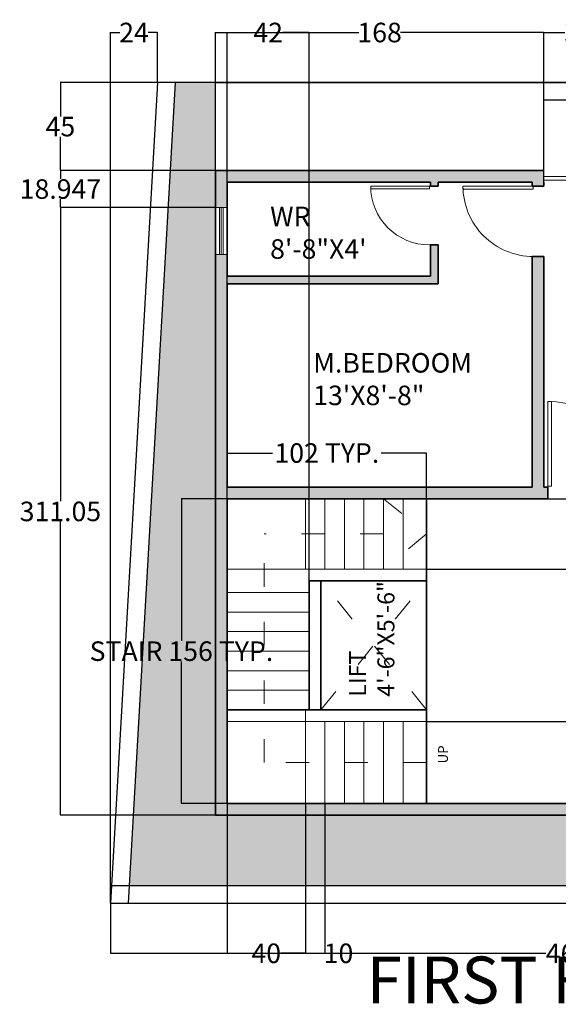
# Model space of a CAD drawing. Units: inches. Extents: x 377 to 1481, y 110 to 618.
# Tile 2 of 3: x 929 to 1205, y 114 to 618. Entities that reach past the tile are written whole.
import ezdxf

# ---------------------------------------------------------------- set-up
doc = ezdxf.new("R2010")
doc.units = ezdxf.units.IN
doc.header["$MEASUREMENT"] = 0
doc.linetypes.add('ACAD_ISO03W100', pattern=[30, 12, -18])
for name, color, linetype, lineweight in [('A-ANNO-DIMS', 2, 'Continuous', 18), ('A-ANNO-TEXT', 7, 'Continuous', 18), ('A-ANNO-TITL', 7, 'Continuous', 35), ('A-AREA-IDEN', 7, 'Continuous', 18), ('A-DOOR', 4, 'Continuous', 18), ('A-FLOR-BALC', 7, 'Continuous', 25), ('A-FLOR-EVTR-SYMB', 7, 'ACAD_ISO03W100', 13), ('A-FLOR-STRS', 7, 'Continuous', 20), ('A-FLOR-STRS-PATH', 7, 'ACAD_ISO03W100', 13), ('A-GLAZ', 4, 'Continuous', 18), ('A-WALL', 7, 'Continuous', 35), ('C-PROP', 7, 'Continuous', 25)]:
    doc.layers.add(name, color=color, linetype=linetype, lineweight=lineweight)
doc.layers.add('A-WALL-PATT', color=251, linetype='Continuous', lineweight=13, true_color=0x636466)
doc.layers.add('L-PLNT-PATT', color=85, linetype='Continuous', lineweight=13, true_color=0x58ba48)
doc.styles.get("Standard").update_dxf_attribs({"font": 'arial.ttf'})
doc.dimstyles.get("Standard").update_dxf_attribs({"dimtxt": 10, "dimasz": 0.18, "dimexe": 0.18, "dimexo": 0.0625, "dimgap": 0.09, "dimtad": 0, "dimtih": 1, "dimtoh": 1, "dimdec": 0, "dimzin": 0, "dimdsep": 46, "dimlunit": 3, "dimtxsty": 'Standard', "dimcen": 0.09, "dimadec": 0, "dimazin": 0, "dimtfac": 1, "dimtdec": 0, "dimtofl": 0, "dimtmove": 0, "dimatfit": 3, "dimfxl": 1, "dimtolj": 1, "dimtzin": 0, "dimarcsym": 0})

# ---------------------------------------------------------------- blocks, each defined once
blk = doc.blocks.new('*U2')
for p, q in [((-40, 0), (-40, 6)), ((0, 0), (0, 6))]:
    blk.add_line(p, q)
blk.add_lwpolyline([(0, 0), (0, -40), (-1.75, -40), (-1.75, 0)], close=True)
blk.add_arc((0, 0), 40, 180, 270)
blk = doc.blocks.new('*U4')
for p, q in [((0, 0), (0, 6)), ((40, 0), (40, 6))]:
    blk.add_line(p, q)
blk.add_lwpolyline([(0, 0), (0, -40), (1.75, -40), (1.75, 0)], close=True)
blk.add_arc((0, 0), 40, 270, 0)
blk = doc.blocks.new('*U5')
for p, q in [((0, 0), (0, 6)), ((40, 0), (40, 6))]:
    blk.add_line(p, q)
blk.add_lwpolyline([(0, 0), (0, -40), (1.75, -40), (1.75, 0)], close=True)
blk.add_arc((0, 0), 40, 270, 0)
blk = doc.blocks.new('WIN-24IN')
for p, q in [((0, 6), (0, 0)), ((24, 6), (24, 0)), ((24, 4), (0, 4)), ((24, 3), (0, 3)), ((24, 2), (0, 2))]:
    blk.add_line(p, q)
blk = doc.blocks.new('STAIR-RETURN-3FLIGHT')
for p, q in [((40, 120), (40, 156)), ((50, 120), (50, 156)), ((60, 120), (60, 156)), ((70, 120), (70, 156)), ((80, 120), (80, 156)), ((90, 120), (90, 156)), ((102, 120), (102, 156)), ((0, 120), (102, 120)), ((0, 108), (42, 108)), ((0, 98), (42, 98)), ((0, 88), (42, 88)), ((0, 78), (42, 78)), ((0, 68), (42, 68)), ((0, 58), (42, 58)), ((40, 0), (40, 48)), ((0, 42), (102, 42)), ((50, 0), (50, 42)), ((60, 0), (60, 42)), ((70, 0), (70, 42)), ((80, 0), (80, 42)), ((90, 0), (90, 42)), ((102, 0), (102, 42))]:
    blk.add_line(p, q)
blk = doc.blocks.new('STAIR-PATH-UP')
for p, q in [((60.99, 117), (60.99, 135)), ((60.99, 135), (82.99, 117)), ((0, 0), (0, 117)), ((60.99, 117), (0, 117)), ((60.99, 119.04), (60.99, 99)), ((82.99, 117), (60.99, 99)), ((82.99, 0), (0, 0))]:
    blk.add_line(p, q)
blk = doc.blocks.new('LIFT-SHAFT-MARK')
for p, q in [((0, 0), (54, 66)), ((54, 0), (0, 66))]:
    blk.add_line(p, q)
blk = doc.blocks.new('*D19')
at = {"layer": 'A-ANNO-DIMS', "color": 0, "lineweight": -2, "transparency": 16777216}
for p, q in [((1035.16, 372.84), (1011.64, 372.84)), ((1011.82, 372.66), (1011.82, 300.1)), ((1011.82, 217.02), (1011.82, 289.58)), ((1035.16, 216.84), (1011.64, 216.84))]:
    blk.add_line(p, q, dxfattribs=at)
at = {"layer": 'A-ANNO-DIMS', "color": 0, "lineweight": 100, "transparency": 16777216}
for points in [[(1011.79, 372.66), (1011.85, 372.66), (1011.82, 372.84)], [(1011.79, 217.02), (1011.85, 217.02), (1011.82, 216.84)]]:
    blk.add_solid(points, dxfattribs=at)
at = {"layer": 'Defpoints', "color": 0, "lineweight": 100, "transparency": 16777216}
for p in [(1011.82, 372.84), (1035.22, 372.84), (1035.22, 216.84)]:
    blk.add_point(p, dxfattribs=at)
at = {"layer": 'A-ANNO-DIMS', "color": 0, "transparency": 16777216, "insert": (1011.82, 294.84), "char_height": 10, "attachment_point": 5}
blk.add_mtext('\\A1;STAIR 156 TYP.', dxfattribs=at)
blk = doc.blocks.new('*D20')
at = {"layer": 'A-ANNO-DIMS', "color": 0, "lineweight": -2, "transparency": 16777216}
for p, q in [((1035.22, 372.9), (1035.22, 396.42)), ((1035.4, 396.24), (1058.38, 396.24)), ((1137.04, 396.24), (1114.07, 396.24)), ((1137.22, 372.9), (1137.22, 396.42))]:
    blk.add_line(p, q, dxfattribs=at)
at = {"layer": 'A-ANNO-DIMS', "color": 0, "lineweight": 100, "transparency": 16777216}
for points in [[(1035.4, 396.27), (1035.4, 396.21), (1035.22, 396.24)], [(1137.04, 396.27), (1137.04, 396.21), (1137.22, 396.24)]]:
    blk.add_solid(points, dxfattribs=at)
at = {"layer": 'Defpoints', "color": 0, "lineweight": 100, "transparency": 16777216}
for p in [(1137.22, 396.24), (1035.22, 372.84), (1137.22, 372.84)]:
    blk.add_point(p, dxfattribs=at)
at = {"layer": 'A-ANNO-DIMS', "color": 0, "transparency": 16777216, "insert": (1086.22, 396.24), "char_height": 10, "attachment_point": 5}
blk.add_mtext('\\A1;102 TYP.', dxfattribs=at)
blk = doc.blocks.new('*D40')
at = {"layer": 'A-ANNO-DIMS', "color": 0, "lineweight": -2, "transparency": 16777216}
for p, q in [((975.57, 165.78), (975.57, 140.01)), ((1443.57, 165.78), (1443.57, 140.01)), ((975.75, 140.19), (1198.22, 140.19)), ((1443.39, 140.19), (1220.92, 140.19))]:
    blk.add_line(p, q, dxfattribs=at)
at = {"layer": 'A-ANNO-DIMS', "color": 0, "lineweight": 100, "transparency": 16777216}
for points in [[(975.75, 140.22), (975.75, 140.16), (975.57, 140.19)], [(1443.39, 140.22), (1443.39, 140.16), (1443.57, 140.19)]]:
    blk.add_solid(points, dxfattribs=at)
at = {"layer": 'Defpoints', "color": 0, "lineweight": 100, "transparency": 16777216}
for p in [(975.57, 165.84), (1443.57, 165.84), (1443.57, 140.19)]:
    blk.add_point(p, dxfattribs=at)
at = {"layer": 'A-ANNO-DIMS', "color": 0, "transparency": 16777216, "insert": (1209.57, 140.19), "char_height": 10, "attachment_point": 5}
blk.add_mtext('\\A1;468', dxfattribs=at)
blk = doc.blocks.new('*D42')
at = {"layer": 'A-ANNO-DIMS', "color": 0, "lineweight": -2, "transparency": 16777216}
for p, q in [((975.57, 165.9), (975.57, 611.67)), ((975.75, 611.49), (980.25, 611.49)), ((999.39, 611.49), (994.89, 611.49)), ((999.57, 585.9), (999.57, 611.67))]:
    blk.add_line(p, q, dxfattribs=at)
at = {"layer": 'A-ANNO-DIMS', "color": 0, "lineweight": 100, "transparency": 16777216}
for points in [[(975.75, 611.52), (975.75, 611.46), (975.57, 611.49)], [(999.39, 611.52), (999.39, 611.46), (999.57, 611.49)]]:
    blk.add_solid(points, dxfattribs=at)
at = {"layer": 'Defpoints', "color": 0, "lineweight": 100, "transparency": 16777216}
for p in [(999.57, 611.49), (999.57, 585.84), (975.57, 165.84)]:
    blk.add_point(p, dxfattribs=at)
at = {"layer": 'A-ANNO-DIMS', "color": 0, "transparency": 16777216, "insert": (987.57, 611.49), "char_height": 10, "attachment_point": 5}
blk.add_mtext('\\A1;24', dxfattribs=at)
blk = doc.blocks.new('*D43')
at = {"layer": 'A-ANNO-DIMS', "color": 0, "lineweight": -2, "transparency": 16777216}
for p, q in [((1029.22, 540.9), (1029.22, 611.67)), ((1029.4, 611.49), (1102.55, 611.49)), ((1197.04, 611.49), (1123.9, 611.49)), ((1197.22, 540.9), (1197.22, 611.67))]:
    blk.add_line(p, q, dxfattribs=at)
at = {"layer": 'A-ANNO-DIMS', "color": 0, "lineweight": 100, "transparency": 16777216}
for points in [[(1029.4, 611.52), (1029.4, 611.46), (1029.22, 611.49)], [(1197.04, 611.52), (1197.04, 611.46), (1197.22, 611.49)]]:
    blk.add_solid(points, dxfattribs=at)
at = {"layer": 'Defpoints', "color": 0, "lineweight": 100, "transparency": 16777216}
for p in [(1197.22, 611.49), (1029.22, 540.84), (1197.22, 540.84)]:
    blk.add_point(p, dxfattribs=at)
at = {"layer": 'A-ANNO-DIMS', "color": 0, "transparency": 16777216, "insert": (1113.22, 611.49), "char_height": 10, "attachment_point": 5}
blk.add_mtext('\\A1;168', dxfattribs=at)
blk = doc.blocks.new('*D46')
at = {"layer": 'A-ANNO-DIMS', "color": 0, "lineweight": -2, "transparency": 16777216}
for p, q in [((1029.16, 521.89), (949.74, 521.89)), ((949.92, 521.71), (949.92, 371.57)), ((949.92, 211.02), (949.92, 361.17)), ((1029.16, 210.84), (949.74, 210.84))]:
    blk.add_line(p, q, dxfattribs=at)
at = {"layer": 'A-ANNO-DIMS', "color": 0, "lineweight": 100, "transparency": 16777216}
for points in [[(949.89, 521.71), (949.95, 521.71), (949.92, 521.89)], [(949.89, 211.02), (949.95, 211.02), (949.92, 210.84)]]:
    blk.add_solid(points, dxfattribs=at)
at = {"layer": 'Defpoints', "color": 0, "lineweight": 100, "transparency": 16777216}
for p in [(949.92, 521.89), (1029.22, 521.89), (1029.22, 210.84)]:
    blk.add_point(p, dxfattribs=at)
at = {"layer": 'A-ANNO-DIMS', "color": 0, "transparency": 16777216, "insert": (949.92, 366.37), "char_height": 10, "attachment_point": 5}
blk.add_mtext('\\A1;311.05', dxfattribs=at)
blk = doc.blocks.new('*D47')
at = {"layer": 'A-ANNO-DIMS', "color": 0, "lineweight": -2, "transparency": 16777216}
for p, q in [((999.51, 585.84), (949.74, 585.84)), ((949.92, 585.66), (949.92, 568.51)), ((949.92, 541.02), (949.92, 558.16)), ((1029.16, 540.84), (949.74, 540.84))]:
    blk.add_line(p, q, dxfattribs=at)
at = {"layer": 'A-ANNO-DIMS', "color": 0, "lineweight": 100, "transparency": 16777216}
for points in [[(949.89, 585.66), (949.95, 585.66), (949.92, 585.84)], [(949.89, 541.02), (949.95, 541.02), (949.92, 540.84)]]:
    blk.add_solid(points, dxfattribs=at)
at = {"layer": 'Defpoints', "color": 0, "lineweight": 100, "transparency": 16777216}
for p in [(949.92, 585.84), (999.57, 585.84), (1029.22, 540.84)]:
    blk.add_point(p, dxfattribs=at)
at = {"layer": 'A-ANNO-DIMS', "color": 0, "transparency": 16777216, "insert": (949.92, 563.34), "char_height": 10, "attachment_point": 5}
blk.add_mtext('\\A1;45', dxfattribs=at)
blk = doc.blocks.new('*D52')
at = {"layer": 'A-ANNO-DIMS', "color": 0, "lineweight": -2, "transparency": 16777216}
for p, q in [((1029.16, 540.84), (949.74, 540.84)), ((949.92, 540.66), (949.92, 536.56)), ((949.92, 522.07), (949.92, 526.17)), ((1029.16, 521.89), (949.74, 521.89))]:
    blk.add_line(p, q, dxfattribs=at)
at = {"layer": 'A-ANNO-DIMS', "color": 0, "lineweight": 100, "transparency": 16777216}
for points in [[(949.89, 540.66), (949.95, 540.66), (949.92, 540.84)], [(949.89, 522.07), (949.95, 522.07), (949.92, 521.89)]]:
    blk.add_solid(points, dxfattribs=at)
at = {"layer": 'Defpoints', "color": 0, "lineweight": 100, "transparency": 16777216}
for p in [(949.92, 540.84), (1029.22, 540.84), (1029.22, 521.89)]:
    blk.add_point(p, dxfattribs=at)
at = {"layer": 'A-ANNO-DIMS', "color": 0, "transparency": 16777216, "insert": (949.92, 531.37), "char_height": 10, "attachment_point": 5}
blk.add_mtext('\\A1;18.947', dxfattribs=at)
blk = doc.blocks.new('*D53')
at = {"layer": 'A-ANNO-DIMS', "color": 0, "lineweight": -2, "transparency": 16777216}
for p, q in [((1197.22, 540.9), (1197.22, 611.67)), ((1197.4, 611.49), (1207.98, 611.49)), ((1233.04, 611.49), (1222.47, 611.49)), ((1233.22, 540.9), (1233.22, 611.67))]:
    blk.add_line(p, q, dxfattribs=at)
at = {"layer": 'A-ANNO-DIMS', "color": 0, "lineweight": 100, "transparency": 16777216}
for points in [[(1197.4, 611.52), (1197.4, 611.46), (1197.22, 611.49)], [(1233.04, 611.52), (1233.04, 611.46), (1233.22, 611.49)]]:
    blk.add_solid(points, dxfattribs=at)
at = {"layer": 'Defpoints', "color": 0, "lineweight": 100, "transparency": 16777216}
for p in [(1233.22, 611.49), (1197.22, 540.84), (1233.22, 540.84)]:
    blk.add_point(p, dxfattribs=at)
at = {"layer": 'A-ANNO-DIMS', "color": 0, "transparency": 16777216, "insert": (1215.22, 611.49), "char_height": 10, "attachment_point": 5}
blk.add_mtext('\\A1;36', dxfattribs=at)
blk = doc.blocks.new('*D54')
at = {"layer": 'A-ANNO-DIMS', "color": 0, "lineweight": -2, "transparency": 16777216}
for p, q in [((1035.22, 216.78), (1035.22, 140.01)), ((1075.22, 216.78), (1075.22, 140.01)), ((1035.4, 140.19), (1047.79, 140.19)), ((1075.04, 140.19), (1062.66, 140.19))]:
    blk.add_line(p, q, dxfattribs=at)
at = {"layer": 'A-ANNO-DIMS', "color": 0, "lineweight": 100, "transparency": 16777216}
for points in [[(1035.4, 140.22), (1035.4, 140.16), (1035.22, 140.19)], [(1075.04, 140.22), (1075.04, 140.16), (1075.22, 140.19)]]:
    blk.add_solid(points, dxfattribs=at)
at = {"layer": 'Defpoints', "color": 0, "lineweight": 100, "transparency": 16777216}
for p in [(1035.22, 216.84), (1075.22, 216.84), (1075.22, 140.19)]:
    blk.add_point(p, dxfattribs=at)
at = {"layer": 'A-ANNO-DIMS', "color": 0, "transparency": 16777216, "insert": (1055.22, 140.19), "char_height": 10, "attachment_point": 5}
blk.add_mtext('\\A1;40', dxfattribs=at)
blk = doc.blocks.new('*D55')
at = {"layer": 'A-ANNO-DIMS', "color": 0, "lineweight": -2, "transparency": 16777216}
for p, q in [((1075.22, 216.78), (1075.22, 140.01)), ((1085.22, 216.78), (1085.22, 140.01)), ((1075.4, 140.19), (1085.04, 140.19)), ((1085.22, 140.19), (1085.4, 140.19))]:
    blk.add_line(p, q, dxfattribs=at)
at = {"layer": 'A-ANNO-DIMS', "color": 0, "lineweight": 100, "transparency": 16777216}
for points in [[(1075.4, 140.22), (1075.4, 140.16), (1075.22, 140.19)], [(1085.04, 140.22), (1085.04, 140.16), (1085.22, 140.19)]]:
    blk.add_solid(points, dxfattribs=at)
at = {"layer": 'Defpoints', "color": 0, "lineweight": 100, "transparency": 16777216}
for p in [(1075.22, 216.84), (1085.22, 216.84), (1085.22, 140.19)]:
    blk.add_point(p, dxfattribs=at)
at = {"layer": 'A-ANNO-DIMS', "color": 0, "transparency": 16777216, "insert": (1092.17, 140.19), "char_height": 10, "attachment_point": 5}
blk.add_mtext('\\A1;10', dxfattribs=at)
blk = doc.blocks.new('*D56')
at = {"layer": 'A-ANNO-DIMS', "color": 0, "lineweight": -2, "transparency": 16777216}
for p, q in [((1137.29, 258.84), (1469.4, 258.84)), ((1469.22, 258.66), (1469.22, 242.95)), ((1469.22, 217.02), (1469.22, 232.73)), ((1137.29, 216.84), (1469.4, 216.84))]:
    blk.add_line(p, q, dxfattribs=at)
at = {"layer": 'A-ANNO-DIMS', "color": 0, "lineweight": 100, "transparency": 16777216}
for points in [[(1469.19, 258.66), (1469.25, 258.66), (1469.22, 258.84)], [(1469.19, 217.02), (1469.25, 217.02), (1469.22, 216.84)]]:
    blk.add_solid(points, dxfattribs=at)
at = {"layer": 'Defpoints', "color": 0, "lineweight": 100, "transparency": 16777216}
for p in [(1137.22, 258.84), (1469.22, 258.84), (1137.22, 216.84)]:
    blk.add_point(p, dxfattribs=at)
at = {"layer": 'A-ANNO-DIMS', "color": 0, "transparency": 16777216, "insert": (1469.22, 237.84), "char_height": 10, "attachment_point": 5}
blk.add_mtext('\\A1;42', dxfattribs=at)
blk = doc.blocks.new('*D57')
at = {"layer": 'A-ANNO-DIMS', "color": 0, "lineweight": -2, "transparency": 16777216}
for p, q in [((1137.29, 372.84), (1469.4, 372.84)), ((1469.22, 372.66), (1469.22, 360.04)), ((1469.22, 337.02), (1469.22, 349.64)), ((1137.29, 336.84), (1469.4, 336.84))]:
    blk.add_line(p, q, dxfattribs=at)
at = {"layer": 'A-ANNO-DIMS', "color": 0, "lineweight": 100, "transparency": 16777216}
for points in [[(1469.19, 372.66), (1469.25, 372.66), (1469.22, 372.84)], [(1469.19, 337.02), (1469.25, 337.02), (1469.22, 336.84)]]:
    blk.add_solid(points, dxfattribs=at)
at = {"layer": 'Defpoints', "color": 0, "lineweight": 100, "transparency": 16777216}
for p in [(1137.22, 372.84), (1469.22, 372.84), (1137.22, 336.84)]:
    blk.add_point(p, dxfattribs=at)
at = {"layer": 'A-ANNO-DIMS', "color": 0, "transparency": 16777216, "insert": (1469.22, 354.84), "char_height": 10, "attachment_point": 5}
blk.add_mtext('\\A1;36', dxfattribs=at)
blk = doc.blocks.new('*D58')
at = {"layer": 'A-ANNO-DIMS', "color": 0, "lineweight": -2, "transparency": 16777216}
for p, q in [((1035.22, 324.9), (1035.22, 611.67)), ((1035.4, 611.49), (1048.82, 611.49)), ((1077.04, 611.49), (1063.63, 611.49)), ((1077.22, 324.9), (1077.22, 611.67))]:
    blk.add_line(p, q, dxfattribs=at)
at = {"layer": 'A-ANNO-DIMS', "color": 0, "lineweight": 100, "transparency": 16777216}
for points in [[(1035.4, 611.52), (1035.4, 611.46), (1035.22, 611.49)], [(1077.04, 611.52), (1077.04, 611.46), (1077.22, 611.49)]]:
    blk.add_solid(points, dxfattribs=at)
at = {"layer": 'Defpoints', "color": 0, "lineweight": 100, "transparency": 16777216}
for p in [(1077.22, 611.49), (1035.22, 324.84), (1077.22, 324.84)]:
    blk.add_point(p, dxfattribs=at)
at = {"layer": 'A-ANNO-DIMS', "color": 0, "transparency": 16777216, "insert": (1056.22, 611.49), "char_height": 10, "attachment_point": 5}
blk.add_mtext('\\A1;42', dxfattribs=at)

msp = doc.modelspace()

# ---------------------------------------------------------------- hatches: boundary and pattern name
at = {"layer": 'A-WALL-PATT'}
h = msp.add_hatch(color=256, dxfattribs=at)
h.dxf.hatch_style = 1
h.paths.add_polyline_path([(1035.2247, 216.8394), (1035.2247, 372.8394), (1137.2247, 372.8394), (1197.2247, 372.8394), (1199.2247, 372.8394), (1199.2247, 378.8394), (1197.2247, 378.8394), (1197.2247, 496.8394), (1191.2247, 496.8394), (1191.2247, 378.8394), (1137.2247, 378.8394), (1035.2247, 378.8394), (1035.2247, 482.8394), (1137.2247, 482.8394), (1143.2247, 482.8394), (1143.2247, 502.8394), (1139.2247, 502.8394), (1139.2247, 486.8394), (1137.2247, 486.8394), (1035.2247, 486.8394), (1035.2247, 497.8925), (1029.2247, 497.8925), (1029.2247, 210.8394), (1258.5701, 210.8394), (1258.5701, 216.8394), (1248.5701, 216.8394), (1248.5701, 300.8394), (1250.5701, 300.8394), (1250.5701, 306.8394), (1248.5701, 306.8394), (1248.5701, 378.8394), (1242.5701, 378.8394), (1242.5701, 216.8394)])
h.paths.add_polyline_path([(1298.5701, 216.8394), (1298.5701, 300.8394), (1300.5689, 300.769), (1300.5689, 306.8394), (1298.5701, 306.8394), (1280.5701, 306.8394), (1280.5701, 300.8394), (1292.5701, 300.8394), (1292.5701, 216.8394), (1282.5701, 216.8394), (1282.5701, 210.8394), (1336.9971, 210.8394), (1336.9971, 216.8394)], flags=17)
h.paths.add_polyline_path([(1360.9971, 216.8394), (1360.9971, 210.8394), (1398.5701, 210.8394), (1398.5701, 540.8394), (1233.2247, 540.8394), (1233.2247, 534.8394), (1392.5701, 534.8394), (1392.5701, 444.8394), (1314.5701, 444.8394), (1314.5701, 438.8394), (1392.5701, 438.8394), (1392.5701, 378.8394), (1314.5701, 378.8394), (1314.5701, 372.8394), (1392.5701, 372.8394), (1392.5701, 306.8394), (1330.6485, 306.8394), (1330.6485, 302.3275, -0.01237335), (1330.6116, 300.8394), (1392.5701, 300.8394), (1392.5701, 216.8394)])
h.paths.add_polyline_path([(1029.2247, 540.8394), (1029.2247, 521.8925), (1035.2247, 521.8925), (1035.2247, 534.8394), (1137.2247, 534.8394), (1139.2247, 534.8394), (1139.2247, 532.8394), (1143.2247, 532.8394), (1143.2247, 534.8394), (1191.2247, 534.8394), (1191.2247, 532.8394), (1197.2247, 532.8394), (1197.2247, 534.8394), (1197.2247, 540.8394), (1137.2247, 540.8394)])
at = {"layer": 'L-PLNT-PATT'}
h = msp.add_hatch(color=256, dxfattribs=at)
h.dxf.hatch_style = 1
h.paths.add_polyline_path([(985.0991, 174.8394), (1434.5701, 174.8394), (1434.5701, 585.8394), (1398.5701, 585.8394), (1398.5701, 540.8394), (1398.5701, 210.8394), (1029.2247, 210.8394), (1029.2247, 540.8394), (1029.2247, 585.8394), (1008.5848, 585.8394)])

# ---------------------------------------------------------------- linework, layer by layer
at = {"layer": 'A-DOOR'}
msp.add_lwpolyline([(1197.2247, 537.8394), (1197.2247, 535.8394), (1215.2247, 535.8394), (1215.2247, 537.8394)], close=True, dxfattribs=at)
at = {"layer": 'A-FLOR-BALC'}
for p, q in [((1029.2247, 540.8394), (1029.2247, 585.8394)), ((1029.2247, 585.8394), (1398.5701, 585.8394)), ((1197.2247, 534.8394), (1197.2247, 585.8394)), ((1293.2247, 576.8394), (1197.2247, 576.8394))]:
    msp.add_line(p, q, dxfattribs=at)
at = {"layer": 'A-WALL'}
for p, q in [((1029.2247, 210.8394), (1029.2247, 540.8394)), ((1029.2247, 540.8394), (1137.2247, 540.8394)), ((1137.2247, 540.8394), (1197.2247, 540.8394)), ((1035.2247, 534.8394), (1137.2247, 534.8394)), ((1035.2247, 486.8394), (1035.2247, 534.8394)), ((1137.2247, 534.8394), (1139.2247, 534.8394)), ((1139.2247, 534.8394), (1139.2247, 532.8394)), ((1143.2247, 532.8394), (1143.2247, 534.8394)), ((1143.2247, 534.8394), (1191.2247, 534.8394)), ((1191.2247, 534.8394), (1191.2247, 532.8394)), ((1197.2247, 532.8394), (1197.2247, 534.8394)), ((1139.2247, 532.8394), (1143.2247, 532.8394)), ((1191.2247, 532.8394), (1197.2247, 532.8394)), ((1139.2247, 486.8394), (1139.2247, 502.8394)), ((1139.2247, 502.8394), (1143.2247, 502.8394)), ((1143.2247, 482.8394), (1143.2247, 502.8394)), ((1191.2247, 378.8394), (1191.2247, 496.8394)), ((1191.2247, 496.8394), (1197.2247, 496.8394)), ((1197.2247, 378.8394), (1197.2247, 496.8394)), ((1035.2247, 486.8394), (1137.2247, 486.8394)), ((1137.2247, 486.8394), (1139.2247, 486.8394)), ((1035.2247, 482.8394), (1137.2247, 482.8394)), ((1035.2247, 378.8394), (1035.2247, 482.8394)), ((1137.2247, 482.8394), (1143.2247, 482.8394)), ((1035.2247, 378.8394), (1137.2247, 378.8394)), ((1137.2247, 378.8394), (1191.2247, 378.8394)), ((1199.2247, 378.8394), (1197.2247, 378.8394)), ((1199.2247, 372.8394), (1199.2247, 378.8394)), ((1035.2247, 372.8394), (1137.2247, 372.8394)), ((1035.2247, 336.8394), (1035.2247, 372.8394)), ((1035.2247, 216.8394), (1035.2247, 372.8394)), ((1035.2247, 372.8394), (1137.2247, 372.8394)), ((1137.2247, 216.8394), (1137.2247, 372.8394)), ((1137.2247, 372.8394), (1197.2247, 372.8394)), ((1197.2247, 372.8394), (1199.2247, 372.8394)), ((1035.2247, 264.8394), (1035.2247, 330.8394)), ((1077.2247, 264.8394), (1077.2247, 330.8394)), ((1077.2247, 330.8394), (1137.2247, 330.8394)), ((1083.2247, 264.8394), (1083.2247, 330.8394)), ((1035.2247, 264.8394), (1137.2247, 264.8394)), ((1035.2247, 216.8394), (1035.2247, 258.8394)), ((1035.2247, 216.8394), (1242.5701, 216.8394)), ((1100.8436, 216.8394), (1202.8436, 216.8394)), ((1029.2247, 210.8394), (1398.5701, 210.8394))]:
    msp.add_line(p, q, dxfattribs=at)
at = {"layer": 'C-PROP'}
for p, q in [((999.5701, 585.8394), (975.5701, 165.8394)), ((1008.5848, 585.8394), (984.5848, 165.8394)), ((1443.5701, 585.8394), (999.5701, 585.8394)), ((976.0844, 174.8394), (1434.5701, 174.8394)), ((975.5701, 165.8394), (1443.5701, 165.8394))]:
    msp.add_line(p, q, dxfattribs=at)

# ---------------------------------------------------------------- block references
at = {"layer": 'A-DOOR'}
for name, p, xscale, yscale, zscale, rotation in [('*U5', (1138.7156, 532.8394), 0.7515245747146567, 0.7515245747146567, 0.7515245747146567, 270), ('*U4', (1191.8294, 532.8394), 0.8992245359782607, 0.8992245359782607, 0.8992245359782607, 270), ('*U2', (1199.2247, 379.3372), 1.082974319922984, 1.082974319922984, 1.082974319922984, 180)]:
    msp.add_blockref(name, p, dxfattribs=dict(at, xscale=xscale, yscale=yscale, zscale=zscale, rotation=rotation))
at = {"layer": 'A-FLOR-EVTR-SYMB'}
msp.add_blockref('LIFT-SHAFT-MARK', (1083.2244, 264.839), dxfattribs=at)
at = {"layer": 'A-FLOR-STRS'}
msp.add_blockref('STAIR-RETURN-3FLIGHT', (1035.2244, 216.839), dxfattribs=at)
at = {"layer": 'A-FLOR-STRS-PATH'}
msp.add_blockref('STAIR-PATH-UP', (1054.2354, 237.839), dxfattribs=at)
at = {"layer": 'A-GLAZ', "rotation": 269.9999999999998}
msp.add_blockref('WIN-24IN', (1029.2243, 521.8926), dxfattribs=at)

# ---------------------------------------------------------------- texts
at = {"layer": 'A-ANNO-TEXT', "insert": (1143.1324, 237.3672), "char_height": 5, "attachment_point": 1, "rotation": 90}
msp.add_mtext_dynamic_manual_height_columns('UP', width=12.2867, gutter_width=1, heights=[0], dxfattribs=at)
at = {"layer": 'A-ANNO-TITL', "insert": (1106.512, 138.5114), "char_height": 24, "attachment_point": 1}
msp.add_mtext_dynamic_manual_height_columns('{\\fTimes New Roman|b0|i0|c0|p18;FIRST FLOOR}', width=313.042105, gutter_width=1, heights=[94.306], dxfattribs=at)
at = {"layer": 'A-AREA-IDEN', "char_height": 10, "attachment_point": 1}
for s, insert in [('WR\\P8\'-8"X4\'', (1057.2093, 522.3535)), ('M.BEDROOM\\P13\'X8\'-8"', (1079.2511, 447.4215))]:
    msp.add_mtext_dynamic_manual_height_columns(s, width=70.118363, gutter_width=1, heights=[0], dxfattribs=dict(at, insert=insert))
at = {"layer": 'A-AREA-IDEN', "insert": (1097.591, 271.505), "char_height": 8.699523, "attachment_point": 1, "rotation": 90}
msp.add_mtext_dynamic_manual_height_columns('LIFT\\P4\'-6"X5\'-6"', width=60.999629, gutter_width=0.87, heights=[0], dxfattribs=at)

# ---------------------------------------------------------------- dimensions: what is measured, and where the dimension line sits
at = {"layer": 'A-ANNO-DIMS'}
for base, p1, p2, picture, middle in [((999.5701, 611.4894), (975.5701, 165.8394), (999.5701, 585.8394), '*D42', (987.5701, 611.4894)), ((1197.2247, 611.4894), (1029.2247, 540.8394), (1197.2247, 540.8394), '*D43', (1113.2247, 611.4894)), ((1077.2247, 611.4894), (1035.2247, 324.8394), (1077.2247, 324.8394), '*D58', (1056.2247, 611.4894)), ((1233.2247, 611.4894), (1197.2247, 540.8394), (1233.2247, 540.8394), '*D53', (1215.2247, 611.4894)), ((1075.2247, 140.1894), (1035.2247, 216.8394), (1075.2247, 216.8394), '*D54', (1055.2247, 140.1894)), ((1085.2247, 140.1894), (1075.2247, 216.8394), (1085.2247, 216.8394), '*D55', (1092.1693, 140.1894)), ((1443.5701, 140.1894), (975.5701, 165.8394), (1443.5701, 165.8394), '*D40', (1209.5701, 140.1894))]:
    dim = msp.add_linear_dim(base=base, p1=p1, p2=p2, dimstyle='Standard', override={"dimdec": 0, "dimlfac": 1, "dimrnd": 0, "dimzin": 0, "dimdsep": 46, "dimlunit": 2}, dxfattribs=at)
    dim.commit()
    dim.dimension.update_dxf_attribs({"geometry": picture, "text_midpoint": middle})
for base, p1, p2, override, picture, middle in [((949.9201, 585.8394), (1029.2247, 540.8394), (999.5701, 585.8394), {"dimdec": 0, "dimlfac": 1, "dimrnd": 0, "dimzin": 0, "dimdsep": 46, "dimlunit": 2}, '*D47', (949.9201, 563.3394)), ((949.9201, 540.8394), (1029.2247, 521.8925), (1029.2247, 540.8394), {"dimdec": 3, "dimlfac": 1, "dimrnd": 0, "dimzin": 0, "dimdsep": 46, "dimlunit": 2}, '*D52', (949.9201, 531.3659)), ((949.9201, 521.8925), (1029.2247, 210.8394), (1029.2247, 521.8925), {"dimdec": 2, "dimlfac": 1, "dimrnd": 0, "dimzin": 0, "dimdsep": 46, "dimlunit": 2}, '*D46', (949.9201, 366.3659)), ((1469.2201, 372.8394), (1137.2247, 336.8394), (1137.2247, 372.8394), {"dimdec": 0, "dimlfac": 1, "dimrnd": 0, "dimzin": 0, "dimdsep": 46, "dimlunit": 2}, '*D57', (1469.2201, 354.8394)), ((1469.2201, 258.8394), (1137.2247, 216.8394), (1137.2247, 258.8394), {"dimdec": 0, "dimlfac": 1, "dimrnd": 0, "dimzin": 0, "dimdsep": 46, "dimlunit": 2}, '*D56', (1469.2201, 237.8394))]:
    dim = msp.add_linear_dim(base=base, p1=p1, p2=p2, angle=90, dimstyle='Standard', override=override, dxfattribs=at)
    dim.commit()
    dim.dimension.update_dxf_attribs({"geometry": picture, "text_midpoint": middle})
dim = msp.add_linear_dim(base=(1137.2247, 396.2394), p1=(1035.2247, 372.8394), p2=(1137.2247, 372.8394), text='<> TYP.', dimstyle='Standard', override={"dimdec": 0, "dimlfac": 1, "dimrnd": 0, "dimzin": 0, "dimdsep": 46, "dimlunit": 2}, dxfattribs=at)
dim.commit()
dim.dimension.update_dxf_attribs({"geometry": '*D20', "text_midpoint": (1086.2247, 396.2394)})
dim = msp.add_linear_dim(base=(1011.8247, 372.8394), p1=(1035.2247, 216.8394), p2=(1035.2247, 372.8394), angle=90, text='STAIR <> TYP.', dimstyle='Standard', override={"dimdec": 0, "dimlfac": 1, "dimrnd": 0, "dimzin": 0, "dimdsep": 46, "dimlunit": 2}, dxfattribs=at)
dim.commit()
dim.dimension.update_dxf_attribs({"geometry": '*D19', "text_midpoint": (1011.8247, 294.8394)})

doc.saveas('drawing.dxf')
